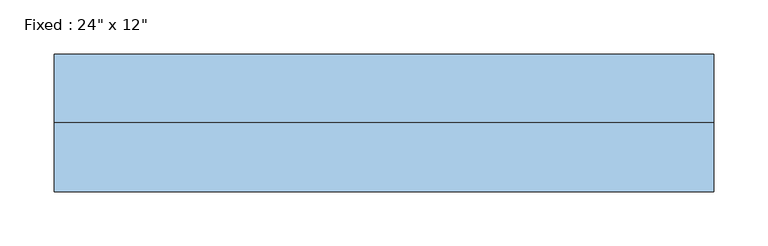
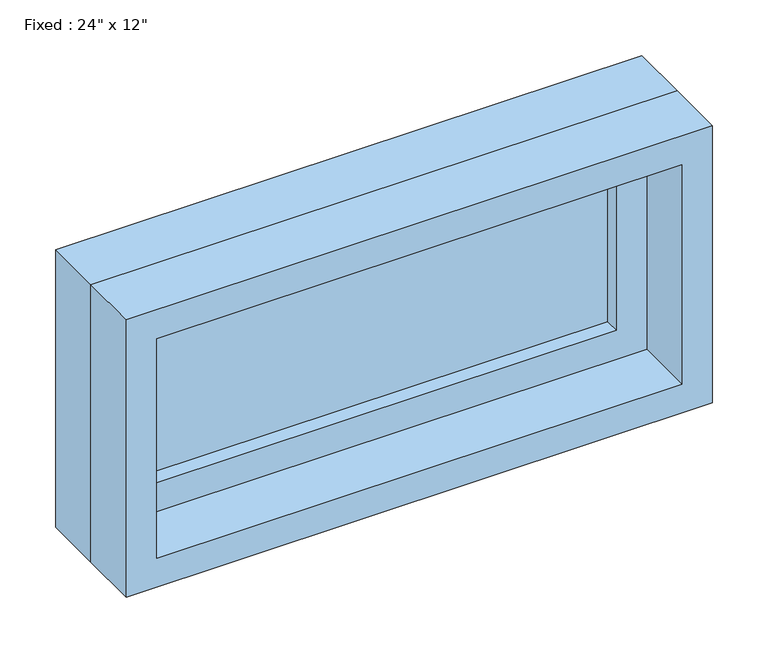
"""IFC4 building model written with IfcOpenShell, lengths in millimetres: window geometry."""

from ifc_helpers import new_model, si_unit, frame, origin, place, context, project, spatial, polyline, outline, extrude, source, transform, mapped, element, save


def window_4c2727af(model_context):
    return source(origin(), model_context, "Body", "SweptSolid", [
        extrude(outline(polyline([(203.2, 15.875), (-279.4, 15.875), (-279.4, 28.575), (203.2, 28.575), (203.2, 15.875)])), frame((0.0, 0.0, 977.9), z_axis=(0.0, 0.0, 1.0), x_axis=(1.0, 0.0, 0.0)), (0.0, 0.0, 1.0), 177.8),
        extrude(outline(polyline([(1200.15, -323.85), (933.45, -323.85), (933.45, 247.65), (1200.15, 247.65), (1200.15, -323.85)]), holes=[polyline([(1155.7, -279.4), (1155.7, 203.2), (977.9, 203.2), (977.9, -279.4), (1155.7, -279.4)])]), frame((0.0, 0.0, 0.0), z_axis=(0.0, 1.0, 0.0), x_axis=(0.0, 0.0, 1.0)), (0.0, 0.0, 1.0), 44.45),
        extrude(outline(polyline([(1219.2, -342.9), (914.4, -342.9), (914.4, 266.7), (1219.2, 266.7), (1219.2, -342.9)]), holes=[polyline([(1187.45, -311.15), (1187.45, 234.95), (946.15, 234.95), (946.15, -311.15), (1187.45, -311.15)])]), frame((0.0, -63.5, 0.0), z_axis=(0.0, 1.0, 0.0), x_axis=(0.0, 0.0, 1.0)), (0.0, 0.0, 1.0), 63.5),
        extrude(outline(polyline([(1219.2, 266.7), (1219.2, -342.9), (914.4, -342.9), (914.4, 266.7), (1219.2, 266.7)]), holes=[polyline([(1200.15, 247.65), (933.45, 247.65), (933.45, -323.85), (1200.15, -323.85), (1200.15, 247.65)])]), frame((0.0, 0.0, 0.0), z_axis=(0.0, 1.0, 0.0), x_axis=(0.0, 0.0, 1.0)), (0.0, 0.0, 1.0), 63.5),
    ])


if __name__ == "__main__":
    model = new_model("IFC4")
    model_context = context("Model", 3, world=origin())
    ifc_project = project(units=[si_unit("LENGTHUNIT", "METRE", prefix="MILLI")], contexts=[model_context])
    site = spatial("IfcSite", under=ifc_project)
    building = spatial("IfcBuilding", under=site)
    placement = place(None, origin())
    window_shape = window_4c2727af(model_context)
    element("IfcWindow", 1, ObjectType="Fixed : 24\" x 12\"", at=placement, inside=building, context=model_context, shape_type="MappedRepresentation", body=[
        mapped(window_shape, transform((0.0, 0.0, 0.0), x_axis=(1.0, 0.0, 0.0), y_axis=(0.0, 1.0, 0.0), z_axis=(0.0, 0.0, 1.0))),
    ])
    save(model, "model.ifc")

# Revit data of these elements
# Type "Fixed : 24\" x 12\""
#   Type Mark = "4"
#   Construction Type Id = "GSP4R"
#   Assembly Code = "B2020100"
#   Analytic Construction = "1/8 in Pilkington single glazing"
#   Visual Light Transmittance = 0.9
#   Solar Heat Gain Coefficient = 0.78
#   Heat Transfer Coefficient (U) = 0.6496 BTU/(h·ft²·°F)
#   Height = 1' - 0"
#   Default Sill Height = 3' - 0"
#   Width = 2' - 0"
#   Window Inset = 0' - 0 3/4"
#   Define Thermal Properties by = 1
#   Define Thermal Properties by = 1
#   Glass Pane Material = Glass
#   Sash Material = Sash
#   Wall Closure = (empty or 0)
# Element 1 (IfcWindow, "Fixed : 24\" x 12\"")
#   Materials on its faces: "Sash", "Glass"
# Materials
#   "Glass": class "Glass", colour RGB 0 128 192, transparency 0.75, Description = "Soda Lime Glass", Cost = 0
#   "Sash": class "Wood", colour RGB 224 178 126, transparency 0, Cost = 0
